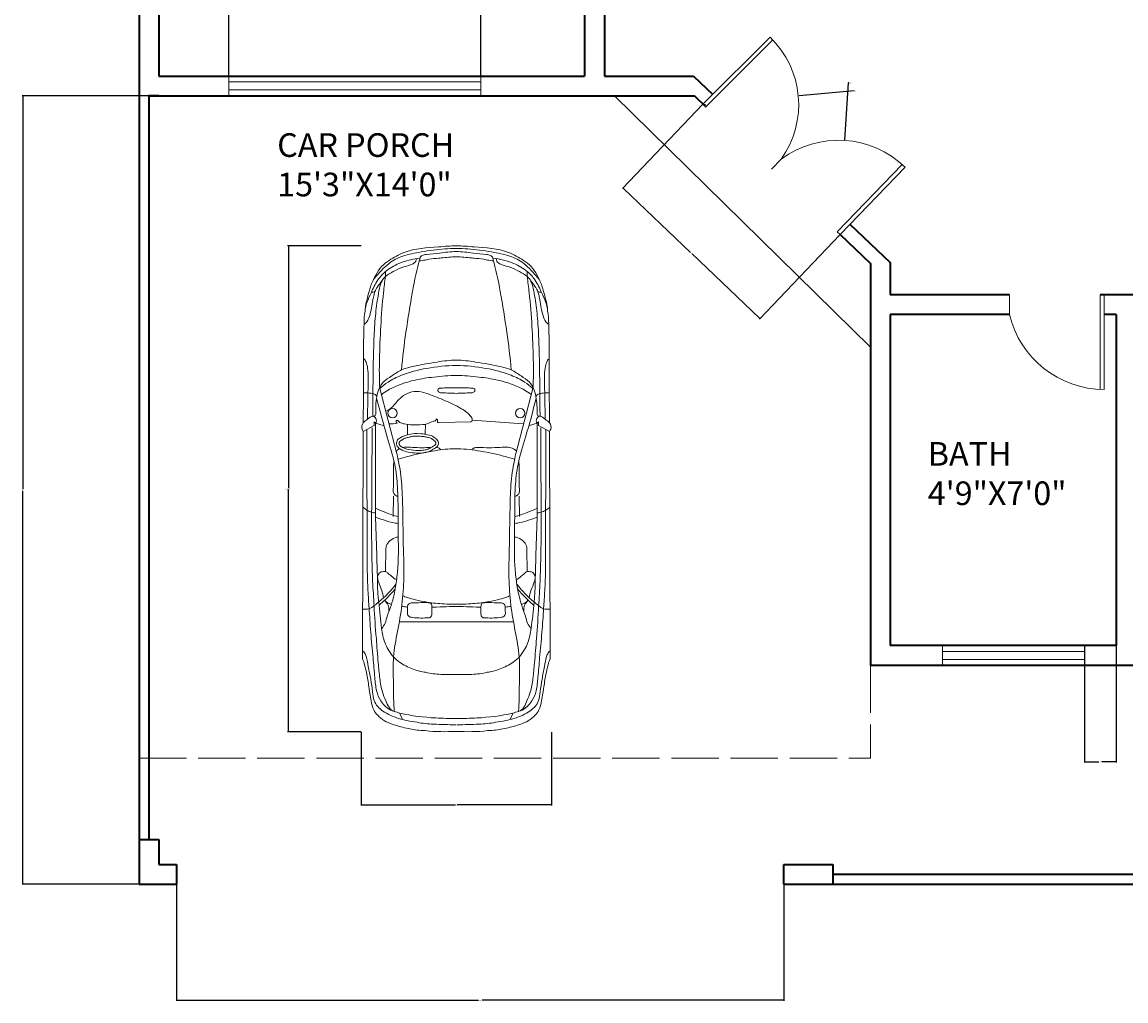
# Model space of a CAD drawing. Units: inches. Extents: x 40921 to 41493, y 89872 to 90511.
# Tile 1 of 4: x 40921 to 41201, y 89872 to 90120. Entities that reach past the tile are written whole.
import ezdxf

# ---------------------------------------------------------------- set-up
doc = ezdxf.new("R2010")
doc.units = ezdxf.units.IN
doc.header["$MEASUREMENT"] = 0
doc.linetypes.add('ACAD_ISO02W100', pattern=[15, 12, -3])
for name, color, linetype, lineweight in [('A-ANNO-DIMS', 2, 'Continuous', 18), ('A-AREA-IDEN', 7, 'Continuous', 18), ('A-DOOR', 3, 'Continuous', 20), ('A-EQPM-VEHC', 8, 'Continuous', 13), ('A-FLOR-STRS', 7, 'Continuous', 18), ('A-GLAZ', 4, 'Continuous', 18), ('A-ROOF-OVHD', 8, 'ACAD_ISO02W100', 13), ('A-WALL', 7, 'Continuous', 35)]:
    doc.layers.add(name, color=color, linetype=linetype, lineweight=lineweight)
doc.styles.get("Standard").update_dxf_attribs({"font": 'arial.ttf'})
doc.dimstyles.get("Standard").update_dxf_attribs({"dimtxt": 0.18, "dimasz": 0.18, "dimexe": 0.18, "dimexo": 0.0625, "dimgap": 0.09, "dimtad": 0, "dimtih": 1, "dimtoh": 1, "dimdec": 4, "dimzin": 0, "dimdsep": 46, "dimtxsty": 'Standard', "dimcen": 0.09, "dimadec": 0, "dimazin": 0, "dimtfac": 1, "dimtdec": 4, "dimtofl": 0, "dimtmove": 0, "dimatfit": 3, "dimfxl": 1, "dimtolj": 1, "dimtzin": 0, "dimarcsym": 0})

# ---------------------------------------------------------------- blocks, each defined once
blk = doc.blocks.new('A$C242571DA')
for p, q in [((1714, 1733), (3817, 1740)), ((1638, 1619), (1625, 1632)), ((1625, 1632), (1660, 1632)), ((1660, 1632), (1714, 1733)), ((1682, 1652), (2695, 1655)), ((1700, 1699), (2985, 1696)), ((1317, 1580), (1910, 1425)), ((1638, 1619), (2503, 1619)), ((1660, 1548), (1638, 1619)), ((2503, 1619), (2862, 1608)), ((1644, 1489), (1610, 1020)), ((2312, 1454), (2501, 1457)), ((3007, 1527), (2808, 1525)), ((3475, 1401), (3475, 843)), ((4315, 1398), (4377, 1370)), ((1626, 1007), (1633, 720)), ((3475, 346), (3475, 904)), ((1740, 585), (1649, 587)), ((1746, 421), (1649, 421)), ((1317, 167), (1910, 322)), ((4315, 349), (4377, 376)), ((2312, 292), (2501, 290)), ((3007, 220), (2808, 222)), ((1638, 128), (1625, 115)), ((1625, 115), (1660, 115)), ((1660, 199), (1638, 128)), ((1638, 128), (2503, 128)), ((1660, 115), (1714, 14)), ((2503, 128), (2862, 139)), ((1682, 95), (2695, 91)), ((1700, 47), (2985, 51)), ((1714, 14), (3817, 7))]:
    blk.add_line(p, q)
for centre in [(1546, 1463), (1546, 284)]:
    blk.add_ellipse(centre, major_axis=(0, 42.9), ratio=0.983266, start_param=4.712389, end_param=10.995574)
for points, knots in [([(605, 1716), (642, 1723), (789, 1729), (1039, 1732), (1344, 1730), (1542, 1733), (1634, 1734)], [0, 0, 0, 0, 0.114897, 0.437061, 0.754269, 1.029686, 1.029686, 1.029686, 1.029686]), ([(1714, 1733), (1708, 1738), (1683, 1753), (1629, 1741), (1606, 1691), (1562, 1652), (1594, 1610), (1628, 1608), (1638, 1619)], [0, 0, 0, 0, 0.024864, 0.0846267, 0.1362471, 0.1900683, 0.2245199, 0.2681841, 0.2681841, 0.2681841, 0.2681841]), ([(2415, 1735), (2425, 1723), (2447, 1699), (2461, 1658), (2468, 1629), (2468, 1616)], [1.808086, 1.808086, 1.808086, 1.808086, 2.918874, 4.131288, 5.10151, 5.10151, 5.10151, 5.10151]), ([(3357, 1739), (3355, 1719), (3361, 1678), (3324, 1632), (3255, 1544), (3187, 1476), (3125, 1432)], [0, 0, 0, 0, 0.0597371, 0.1139981, 0.1672498, 0.3938869, 0.3938869, 0.3938869, 0.3938869]), ([(3745, 1737), (3749, 1730), (3764, 1717), (3811, 1699), (3895, 1687), (4003, 1663), (4108, 1649), (4196, 1638), (4259, 1603), (4302, 1550), (4340, 1484), (4365, 1408), (4390, 1324), (4398, 1267), (4402, 1235)], [0, 0, 0, 0, 0.0219205, 0.0572122, 0.1522539, 0.2718866, 0.3894011, 0.4710097, 0.5346344, 0.5986698, 0.6733118, 0.758696, 0.8351341, 0.9293726, 0.9293726, 0.9293726, 0.9293726]), ([(3817, 1740), (3833, 1730), (3883, 1718), (3973, 1695), (4085, 1680), (4194, 1663), (4281, 1644), (4344, 1598), (4390, 1540), (4427, 1449), (4458, 1337), (4476, 1233), (4478, 1175), (4479, 1162)], [0, 0, 0, 0, 0.056668, 0.14946, 0.28161, 0.392935, 0.481686, 0.542967, 0.622845, 0.69797, 0.833643, 0.965665, 1.00577, 1.00577, 1.00577, 1.00577]), ([(0, 873), (0, 928), (16, 1089), (26, 1310), (121, 1476), (189, 1569), (273, 1623), (370, 1666), (483, 1695), (561, 1715), (605, 1716)], [0, 0, 0, 0, 0.16039, 0.479033, 0.632967, 0.722015, 0.817474, 0.927562, 1.03733, 1.167094, 1.167094, 1.167094, 1.167094]), ([(311, 1637), (282, 1614), (230, 1570), (149, 1486), (85, 1361), (60, 1219), (33, 1054), (25, 945), (25, 873)], [0, 0, 0, 0, 0.1095129, 0.2035347, 0.3452507, 0.5161382, 0.6275464, 0.8383798, 0.8383798, 0.8383798, 0.8383798]), ([(605, 1716), (546, 1714), (449, 1665), (321, 1611), (225, 1521), (147, 1391), (122, 1275), (114, 1209)], [0, 0, 0, 0, 0.1772572, 0.3124951, 0.4151678, 0.5597243, 0.7575412, 0.7575412, 0.7575412, 0.7575412]), ([(427, 1657), (429, 1647), (427, 1625), (400, 1617), (368, 1594), (328, 1565), (272, 1524), (237, 1452), (196, 1377), (184, 1315), (170, 1280), (157, 1254), (133, 1244), (119, 1243)], [0, 0, 0, 0, 0.0304541, 0.0502818, 0.0786089, 0.1479133, 0.1986294, 0.2831705, 0.3780326, 0.4523267, 0.4667809, 0.4902599, 0.5347198, 0.5347198, 0.5347198, 0.5347198]), ([(324, 1558), (345, 1572), (400, 1585), (516, 1607), (680, 1626), (885, 1636), (1117, 1642), (1346, 1644), (1505, 1645), (1574, 1646)], [0, 0, 0, 0, 0.076148, 0.165903, 0.355672, 0.569871, 0.782325, 1.050047, 1.257936, 1.257936, 1.257936, 1.257936]), ([(723, 1727), (721, 1715), (694, 1690), (643, 1672), (574, 1655), (508, 1647), (455, 1635), (429, 1627), (417, 1624)], [0, 0, 0, 0, 0.034703, 0.0959761, 0.1659336, 0.2471559, 0.2929944, 0.3295918, 0.3295918, 0.3295918, 0.3295918]), ([(1044, 1729), (1049, 1718), (1081, 1704), (1139, 1688), (1238, 1686), (1395, 1691), (1522, 1692), (1601, 1693)], [0, 0, 0, 0, 0.0364992, 0.0923739, 0.1867837, 0.3273982, 0.5667068, 0.5667068, 0.5667068, 0.5667068]), ([(1357, 1732), (1357, 1713), (1360, 1679), (1364, 1630), (1383, 1614), (1391, 1607)], [0, 0, 0, 0, 1.462159, 2.651105, 3.386321, 3.386321, 3.386321, 3.386321]), ([(1574, 1646), (1573, 1638), (1574, 1622), (1560, 1619), (1555, 1618)], [0, 0, 0, 0, 0.02274132, 0.03717479, 0.03717479, 0.03717479, 0.03717479]), ([(2695, 1655), (2830, 1655), (3041, 1651), (3351, 1631), (3527, 1623), (3627, 1612)], [0, 0, 0, 0, 0.4042759, 0.6333827, 0.9326252, 0.9326252, 0.9326252, 0.9326252]), ([(2985, 1696), (3051, 1696), (3172, 1691), (3367, 1678), (3575, 1664), (3788, 1644), (3968, 1628), (4104, 1617), (4204, 1578), (4272, 1519), (4301, 1452), (4342, 1305), (4362, 1111), (4367, 937), (4367, 873)], [0, 0, 0, 0, 0.198873, 0.363323, 0.587433, 0.823543, 1.004622, 1.129816, 1.230113, 1.320655, 1.388577, 1.443334, 1.771447, 1.958652, 1.958652, 1.958652, 1.958652]), ([(1317, 1580), (1228, 1586), (1036, 1585), (741, 1573), (486, 1553), (333, 1534), (283, 1528)], [0, 0, 0, 0, 0.269375, 0.574535, 0.885339, 1.036319, 1.036319, 1.036319, 1.036319]), ([(1555, 1618), (1528, 1618), (1473, 1620), (1393, 1609), (1318, 1591), (1249, 1545), (1201, 1467), (1143, 1386), (1105, 1240), (1076, 1072), (1056, 932), (1056, 873)], [0, 0, 0, 0, 0.082256, 0.165174, 0.241383, 0.30939, 0.405348, 0.511507, 0.603349, 0.843635, 1.017671, 1.017671, 1.017671, 1.017671]), ([(1317, 1580), (1297, 1556), (1248, 1494), (1178, 1350), (1124, 1137), (1106, 965), (1106, 873)], [0, 0, 0, 0, 0.0947759, 0.2311242, 0.4700259, 0.7400315, 0.7400315, 0.7400315, 0.7400315]), ([(1373, 1563), (1357, 1545), (1322, 1490), (1277, 1386), (1233, 1244), (1211, 1069), (1197, 942), (1197, 873)], [0, 0, 0, 0, 0.0708922, 0.1925846, 0.3348457, 0.5072814, 0.7109928, 0.7109928, 0.7109928, 0.7109928]), ([(3536, 1563), (3520, 1551), (3484, 1526), (3408, 1511), (3323, 1473), (3208, 1445), (3073, 1422), (2867, 1405), (2626, 1413), (2397, 1411), (2201, 1417), (2001, 1438), (1732, 1526), (1528, 1579), (1408, 1611)], [0, 0, 0, 0, 0.05975, 0.126928, 0.230034, 0.336675, 0.482225, 0.641324, 0.954906, 1.203173, 1.330375, 1.542773, 1.802261, 2.175545, 2.175545, 2.175545, 2.175545]), ([(2424, 1619), (2442, 1590), (2464, 1519), (2495, 1451), (2502, 1411)], [0, 0, 0, 0, 0.1000351, 0.2184418, 0.2184418, 0.2184418, 0.2184418]), ([(2508, 1618), (2521, 1588), (2537, 1527), (2560, 1458), (2563, 1421), (2564, 1411)], [0, 0, 0, 0, 2.528586, 4.711885, 5.408215, 5.408215, 5.408215, 5.408215]), ([(2862, 1608), (2921, 1607), (3047, 1601), (3191, 1602), (3357, 1584), (3498, 1571), (3623, 1549), (3664, 1533)], [0, 0, 0, 0, 0.1783018, 0.3787173, 0.431954, 0.6762374, 0.8077184, 0.8077184, 0.8077184, 0.8077184]), ([(3248, 1545), (3227, 1550), (3176, 1562), (3114, 1593), (3053, 1605), (3010, 1579), (3010, 1545), (3010, 1516), (3034, 1500), (3053, 1465), (3079, 1444), (3084, 1424)], [0, 0, 0, 0, 0.0655106, 0.1550445, 0.2094604, 0.2438604, 0.287164, 0.3001388, 0.3275984, 0.3616951, 0.4200969, 0.4200969, 0.4200969, 0.4200969]), ([(3319, 1587), (3303, 1568), (3257, 1517), (3207, 1467), (3171, 1440)], [0, 0, 0, 0, 1.868162, 5.271297, 5.271297, 5.271297, 5.271297]), ([(3275, 1533), (3288, 1528), (3300, 1505), (3308, 1482), (3312, 1473)], [0, 0, 0, 0, 0.983949, 1.771691, 1.771691, 1.771691, 1.771691]), ([(3372, 1495), (3354, 1497), (3316, 1495), (3292, 1526), (3275, 1533)], [0, 0, 0, 0, 0.0535488, 0.1060573, 0.1060573, 0.1060573, 0.1060573]), ([(3627, 1612), (3702, 1609), (3826, 1597), (3991, 1583), (4112, 1562), (4212, 1523), (4290, 1488), (4301, 1448)], [0, 0, 0, 0, 0.2277977, 0.3719478, 0.4996814, 0.5863441, 0.709615, 0.709615, 0.709615, 0.709615]), ([(3664, 1533), (3687, 1526), (3735, 1502), (3817, 1445), (3884, 1343), (3925, 1240), (3937, 1177), (3940, 1158)], [0, 0, 0, 0, 0.0720749, 0.1581284, 0.2958089, 0.4262456, 0.4842292, 0.4842292, 0.4842292, 0.4842292]), ([(1910, 1425), (1933, 1419), (1996, 1408), (2094, 1386), (2212, 1377), (2419, 1367), (2705, 1366), (3033, 1354), (3316, 1371), (3559, 1416), (3789, 1462), (4029, 1453), (4196, 1455), (4293, 1448), (4301, 1448)], [0, 0, 0, 0, 0.073325, 0.188896, 0.303039, 0.425821, 0.811242, 1.159737, 1.41058, 1.660623, 1.899627, 2.11145, 2.377727, 2.401703, 2.401703, 2.401703, 2.401703]), ([(1997, 1450), (2040, 1455), (2127, 1452), (2220, 1454), (2287, 1457), (2306, 1434), (2313, 1420), (2316, 1414)], [0, 0, 0, 0, 3.267856, 6.568708, 7.399663, 8.099385, 8.621705, 8.621705, 8.621705, 8.621705]), ([(2808, 1525), (2792, 1525), (2752, 1520), (2711, 1473), (2690, 1431), (2691, 1410)], [0, 0, 0, 0, 0.0486628, 0.1144515, 0.1777721, 0.1777721, 0.1777721, 0.1777721]), ([(114, 1209), (215, 1239), (443, 1285), (788, 1339), (1030, 1371), (1146, 1379)], [0, 0, 0, 0, 0.317374, 0.69576, 1.04714, 1.04714, 1.04714, 1.04714]), ([(1898, 1426), (1889, 1421), (1871, 1397), (1856, 1345), (1868, 1234), (1864, 1132), (1863, 1038), (1877, 1022), (1885, 1016)], [0, 0, 0, 0, 0.842998, 2.122875, 3.997599, 9.174838, 10.012722, 10.751336, 10.751336, 10.751336, 10.751336]), ([(1970, 1407), (1960, 1370), (1927, 1259), (1891, 1078), (1874, 933), (1874, 864)], [0, 0, 0, 0, 0.1139079, 0.3411539, 0.543502, 0.543502, 0.543502, 0.543502]), ([(3232, 1368), (3241, 1356), (3253, 1316), (3272, 1241), (3298, 1128), (3311, 975), (3311, 858), (3312, 794)], [0, 0, 0, 0, 0.0451009, 0.1211996, 0.2308505, 0.385263, 0.5739042, 0.5739042, 0.5739042, 0.5739042]), ([(3295, 1175), (3295, 1207), (3300, 1250), (3298, 1304), (3326, 1329), (3364, 1321), (3399, 1329), (3422, 1316), (3431, 1298), (3439, 1234), (3440, 1174), (3435, 1112), (3419, 1102), (3396, 1099), (3363, 1101), (3331, 1097), (3299, 1108), (3297, 1140), (3295, 1161), (3295, 1175)], [0, 0, 0, 0, 0.0969044, 0.1295913, 0.1506192, 0.1985921, 0.2360698, 0.2557908, 0.2719711, 0.2929882, 0.44406, 0.4519132, 0.4720918, 0.4918599, 0.5228758, 0.5707096, 0.5892096, 0.6145759, 0.654681, 0.654681, 0.654681, 0.654681]), ([(4402, 1235), (4412, 1185), (4422, 1066), (4424, 946), (4424, 878)], [0, 0, 0, 0, 0.1502861, 0.3522699, 0.3522699, 0.3522699, 0.3522699]), ([(114, 1209), (103, 1207), (84, 1188), (76, 1122), (68, 1017), (53, 925), (53, 873)], [0, 0, 0, 0, 0.0314754, 0.0702057, 0.1915753, 0.3439346, 0.3439346, 0.3439346, 0.3439346]), ([(136, 1213), (139, 1212), (138, 1193), (133, 1168), (119, 1112), (116, 1059), (109, 975), (102, 920), (102, 873)], [0, 0, 0, 0, 0.0114788, 0.0403472, 0.0875838, 0.1755608, 0.1991501, 0.3369659, 0.3369659, 0.3369659, 0.3369659]), ([(3940, 1158), (3950, 1111), (3964, 1016), (3960, 921), (3960, 873)], [0, 0, 0, 0, 0.140379, 0.2808468, 0.2808468, 0.2808468, 0.2808468]), ([(1311, 873), (1311, 902), (1309, 951), (1315, 1002), (1314, 1039), (1332, 1045), (1346, 1044), (1357, 1029), (1359, 970), (1362, 918), (1363, 873)], [0, 0, 0, 0, 0.0857277, 0.1381048, 0.1641986, 0.1769751, 0.1890325, 0.2028129, 0.2286049, 0.3592554, 0.3592554, 0.3592554, 0.3592554]), ([(1626, 1007), (1623, 1013), (1603, 1029), (1559, 995), (1523, 952), (1480, 878), (1431, 774), (1385, 658), (1344, 551), (1343, 462), (1380, 387), (1428, 330), (1480, 295), (1510, 257), (1525, 233), (1528, 222)], [0, 0, 0, 0, 0.527288, 1.647451, 3.487558, 5.099073, 7.968657, 12.238313, 14.475187, 16.613757, 18.744202, 20.639343, 22.223389, 23.452731, 24.286529, 24.286529, 24.286529, 24.286529]), ([(3339, 1099), (3339, 1095), (3336, 1011), (3333, 926), (3330, 846)], [11.235438, 11.235438, 11.235438, 11.235438, 11.552536, 17.586883, 17.586883, 17.586883, 17.586883]), ([(3232, 379), (3241, 391), (3253, 431), (3272, 506), (3298, 619), (3311, 772), (3311, 888), (3312, 952)], [0, 0, 0, 0, 0.0451009, 0.1211996, 0.2308505, 0.385263, 0.5739042, 0.5739042, 0.5739042, 0.5739042]), ([(0, 873), (0, 819), (16, 658), (26, 437), (121, 270), (189, 178), (273, 124), (370, 80), (483, 52), (561, 32), (605, 31)], [0, 0, 0, 0, 0.16039, 0.479033, 0.632967, 0.722015, 0.817474, 0.927562, 1.03733, 1.167094, 1.167094, 1.167094, 1.167094]), ([(311, 109), (282, 133), (230, 177), (149, 261), (85, 385), (60, 528), (33, 692), (25, 802), (25, 873)], [0, 0, 0, 0, 0.1095129, 0.2035347, 0.3452507, 0.5161382, 0.6275464, 0.8383798, 0.8383798, 0.8383798, 0.8383798]), ([(114, 538), (103, 540), (84, 559), (76, 625), (68, 729), (53, 822), (53, 873)], [0, 0, 0, 0, 0.0314754, 0.0702057, 0.1915753, 0.3439346, 0.3439346, 0.3439346, 0.3439346]), ([(136, 534), (139, 535), (138, 553), (133, 578), (119, 635), (116, 688), (109, 772), (102, 827), (102, 873)], [0, 0, 0, 0, 0.0114788, 0.0403472, 0.0875838, 0.1755608, 0.1991501, 0.3369659, 0.3369659, 0.3369659, 0.3369659]), ([(1555, 129), (1528, 129), (1473, 126), (1393, 138), (1318, 156), (1249, 201), (1201, 280), (1143, 361), (1105, 506), (1076, 674), (1056, 814), (1056, 873)], [0, 0, 0, 0, 0.082256, 0.165174, 0.241383, 0.30939, 0.405348, 0.511507, 0.603349, 0.843635, 1.017671, 1.017671, 1.017671, 1.017671]), ([(1317, 167), (1297, 191), (1248, 252), (1178, 396), (1124, 609), (1106, 782), (1106, 873)], [0, 0, 0, 0, 0.0947759, 0.2311242, 0.4700259, 0.7400315, 0.7400315, 0.7400315, 0.7400315]), ([(1373, 184), (1357, 202), (1322, 257), (1277, 361), (1233, 503), (1211, 677), (1197, 804), (1197, 873)], [0, 0, 0, 0, 0.0708922, 0.1925846, 0.3348457, 0.5072814, 0.7109928, 0.7109928, 0.7109928, 0.7109928]), ([(1311, 873), (1311, 844), (1309, 796), (1315, 745), (1314, 707), (1332, 702), (1346, 703), (1357, 718), (1359, 777), (1362, 829), (1363, 873)], [0, 0, 0, 0, 0.0857277, 0.1381048, 0.1641986, 0.1769751, 0.1890325, 0.2028129, 0.2286049, 0.3592554, 0.3592554, 0.3592554, 0.3592554]), ([(1970, 339), (1960, 377), (1927, 488), (1893, 663), (1874, 802), (1874, 864)], [0, 0, 0, 0, 0.1139079, 0.3411539, 0.5260188, 0.5260188, 0.5260188, 0.5260188]), ([(2985, 51), (3051, 51), (3172, 56), (3367, 69), (3575, 82), (3788, 103), (3968, 119), (4104, 130), (4204, 169), (4272, 227), (4301, 295), (4342, 441), (4362, 636), (4367, 810), (4367, 873)], [0, 0, 0, 0, 0.198873, 0.363323, 0.587433, 0.823543, 1.004622, 1.129816, 1.230113, 1.320655, 1.388577, 1.443334, 1.771447, 1.958652, 1.958652, 1.958652, 1.958652]), ([(3339, 648), (3339, 652), (3336, 736), (3333, 820), (3330, 901)], [11.235438, 11.235438, 11.235438, 11.235438, 11.552536, 17.586883, 17.586883, 17.586883, 17.586883]), ([(3940, 589), (3950, 636), (3964, 730), (3960, 826), (3960, 873)], [0, 0, 0, 0, 0.140379, 0.2808468, 0.2808468, 0.2808468, 0.2808468]), ([(4402, 512), (4412, 561), (4422, 681), (4424, 800), (4424, 869)], [0, 0, 0, 0, 0.1502861, 0.3522699, 0.3522699, 0.3522699, 0.3522699]), ([(1639, 326), (1635, 324), (1629, 318), (1613, 315), (1612, 324), (1613, 330), (1619, 338), (1629, 346), (1638, 366), (1649, 405), (1656, 473), (1656, 543), (1645, 611), (1623, 651), (1615, 684), (1598, 691), (1604, 697), (1610, 700), (1619, 699), (1626, 701), (1638, 699), (1633, 713), (1633, 720)], [0, 0, 0, 0, 0.0138597, 0.0278304, 0.0329137, 0.0379971, 0.0465756, 0.0592704, 0.0762214, 0.1105991, 0.1789801, 0.2766959, 0.3173629, 0.3800771, 0.4110544, 0.4160421, 0.4210284, 0.4277212, 0.4387433, 0.4448131, 0.4508005, 0.4694463, 0.4694463, 0.4694463, 0.4694463]), ([(1863, 686), (1864, 694), (1865, 711), (1877, 724), (1885, 731)], [9.436432, 9.436432, 9.436432, 9.436432, 10.012722, 10.751336, 10.751336, 10.751336, 10.751336]), ([(1740, 585), (1738, 572), (1750, 644), (1766, 664), (1792, 700), (1821, 710), (1853, 704), (1874, 668), (1905, 623), (1916, 557), (1915, 484), (1906, 418), (1885, 363), (1859, 329), (1831, 318), (1811, 323), (1792, 329), (1778, 350), (1753, 386), (1738, 466), (1729, 497), (1742, 598), (1740, 585)], [0, 0, 0, 0, 0.03969, 0.089634, 0.13125, 0.1542862, 0.1797268, 0.2207266, 0.2680991, 0.3447665, 0.4095645, 0.4843001, 0.541515, 0.5817687, 0.6060665, 0.6262474, 0.6436722, 0.6634686, 0.6988791, 0.7758465, 0.8696394, 0.907731, 0.907731, 0.907731, 0.907731]), ([(1765, 587), (1766, 591), (1766, 595), (1769, 606), (1770, 611), (1773, 627), (1776, 633), (1780, 642), (1782, 645), (1786, 651), (1787, 653), (1793, 660), (1797, 666), (1804, 674), (1807, 676), (1811, 679), (1813, 680), (1817, 682), (1819, 683), (1824, 683), (1828, 683), (1832, 682), (1834, 682), (1836, 680), (1838, 679), (1842, 674), (1845, 670), (1850, 662), (1853, 657), (1859, 647), (1862, 643), (1868, 633), (1871, 627), (1877, 616), (1879, 610), (1883, 597), (1884, 591), (1888, 571), (1890, 556), (1891, 527), (1891, 513), (1889, 470), (1885, 441), (1874, 404), (1871, 394), (1863, 379), (1861, 373), (1854, 364), (1851, 359), (1845, 353), (1842, 350), (1836, 346), (1833, 345), (1829, 345), (1828, 345), (1825, 345), (1823, 345), (1818, 346), (1815, 347), (1811, 349), (1809, 349), (1808, 350), (1808, 350), (1807, 351), (1807, 352), (1805, 354), (1803, 356), (1800, 361), (1798, 364), (1795, 368), (1793, 370), (1789, 377), (1787, 381), (1782, 389), (1780, 394), (1777, 403), (1775, 408), (1771, 423), (1768, 434), (1765, 450), (1764, 456), (1761, 467), (1760, 471), (1758, 484), (1757, 493), (1758, 511), (1758, 516), (1759, 528), (1759, 534), (1761, 554), (1763, 571), (1764, 581), (1765, 583), (1765, 585), (1765, 585), (1765, 586), (1765, 587), (1765, 587)], [0.497033, 0.497033, 0.497033, 0.497033, 0.723444, 0.723444, 0.974636, 0.974636, 1.50964, 1.50964, 2.044645, 2.044645, 2.271061, 2.271061, 2.862376, 2.862376, 3.217654, 3.217654, 3.537253, 3.537253, 3.856852, 3.856852, 4.368613, 4.368613, 4.584627, 4.584627, 4.99269, 4.99269, 5.400753, 5.400753, 5.808816, 5.808816, 6.216879, 6.216879, 6.778716, 6.778716, 7.350371, 7.350371, 7.922025, 7.922025, 9.065335, 9.065335, 10.208644, 10.208644, 12.495263, 12.495263, 13.409896, 13.409896, 13.929088, 13.929088, 14.44828, 14.44828, 14.909885, 14.909885, 15.371489, 15.371489, 15.62524, 15.62524, 15.87899, 15.87899, 16.120875, 16.120875, 16.36276, 16.36276, 16.51635, 16.51635, 16.669941, 16.669941, 16.921521, 16.921521, 17.136676, 17.136676, 17.351831, 17.351831, 17.782142, 17.782142, 18.204974, 18.204974, 18.627807, 18.627807, 19.473473, 19.473473, 19.978923, 19.978923, 20.484372, 20.484372, 21.475119, 21.475119, 21.859144, 21.859144, 22.162884, 22.162884, 22.770362, 22.770362, 22.900493, 22.900493, 22.951221, 22.951221, 22.964298, 22.964298, 22.964298, 22.964298]), ([(1864, 379), (1863, 384), (1858, 414), (1867, 502), (1865, 581), (1864, 639)], [1.749253, 1.749253, 1.749253, 1.749253, 2.122875, 3.997599, 8.307432, 8.307432, 8.307432, 8.307432]), ([(3295, 572), (3295, 539), (3300, 497), (3298, 443), (3326, 418), (3364, 426), (3399, 417), (3422, 431), (3431, 449), (3439, 513), (3440, 572), (3435, 635), (3419, 645), (3396, 648), (3363, 646), (3331, 650), (3299, 639), (3297, 606), (3295, 586), (3295, 572)], [0, 0, 0, 0, 0.0969044, 0.1295913, 0.1506192, 0.1985921, 0.2360698, 0.2557908, 0.2719711, 0.2929882, 0.44406, 0.4519132, 0.4720918, 0.4918599, 0.5228758, 0.5707096, 0.5892096, 0.6145759, 0.654681, 0.654681, 0.654681, 0.654681]), ([(605, 31), (546, 32), (449, 82), (321, 136), (225, 226), (147, 356), (122, 472), (114, 538)], [0, 0, 0, 0, 0.1772572, 0.3124951, 0.4151678, 0.5597243, 0.7575412, 0.7575412, 0.7575412, 0.7575412]), ([(114, 538), (215, 508), (443, 462), (788, 408), (1030, 376), (1146, 368)], [0, 0, 0, 0, 0.317374, 0.69576, 1.04714, 1.04714, 1.04714, 1.04714]), ([(3664, 214), (3687, 221), (3735, 244), (3817, 302), (3884, 404), (3925, 507), (3937, 570), (3940, 589)], [0, 0, 0, 0, 0.0720749, 0.1581284, 0.2958089, 0.4262456, 0.4842292, 0.4842292, 0.4842292, 0.4842292]), ([(3745, 10), (3749, 17), (3764, 30), (3811, 48), (3895, 60), (4003, 84), (4108, 98), (4196, 108), (4259, 144), (4302, 197), (4340, 263), (4365, 339), (4390, 422), (4398, 480), (4402, 512)], [0, 0, 0, 0, 0.0219205, 0.0572122, 0.1522539, 0.2718866, 0.3894011, 0.4710097, 0.5346344, 0.5986698, 0.6733118, 0.758696, 0.8351341, 0.9293726, 0.9293726, 0.9293726, 0.9293726]), ([(3817, 7), (3833, 17), (3883, 29), (3973, 52), (4085, 66), (4194, 84), (4281, 102), (4344, 149), (4390, 206), (4427, 298), (4458, 410), (4476, 513), (4478, 572), (4479, 585)], [0, 0, 0, 0, 0.056668, 0.14946, 0.28161, 0.392935, 0.481686, 0.542967, 0.622845, 0.69797, 0.833643, 0.965665, 1.00577, 1.00577, 1.00577, 1.00577]), ([(427, 90), (429, 100), (427, 122), (400, 130), (368, 153), (328, 182), (272, 223), (237, 295), (196, 370), (184, 432), (170, 467), (157, 493), (133, 502), (119, 504)], [0, 0, 0, 0, 0.0304541, 0.0502818, 0.0786089, 0.1479133, 0.1986294, 0.2831705, 0.3780326, 0.4523267, 0.4667809, 0.4902599, 0.5347198, 0.5347198, 0.5347198, 0.5347198]), ([(3536, 184), (3520, 196), (3484, 221), (3408, 236), (3323, 274), (3208, 302), (3073, 325), (2867, 342), (2626, 334), (2397, 336), (2201, 330), (2001, 309), (1732, 221), (1528, 168), (1408, 136)], [0, 0, 0, 0, 0.05975, 0.126928, 0.230034, 0.336675, 0.482225, 0.641324, 0.954906, 1.203173, 1.330375, 1.542773, 1.802261, 2.175545, 2.175545, 2.175545, 2.175545]), ([(1898, 321), (1889, 326), (1881, 337), (1875, 348), (1874, 350)], [0, 0, 0, 0, 0.8429982, 0.9626806, 0.9626806, 0.9626806, 0.9626806]), ([(1910, 322), (1933, 328), (1996, 339), (2094, 361), (2212, 370), (2419, 380), (2705, 380), (3033, 393), (3316, 376), (3559, 331), (3789, 285), (4029, 294), (4196, 292), (4293, 299), (4301, 299)], [0, 0, 0, 0, 0.073325, 0.188896, 0.303039, 0.425821, 0.811242, 1.159737, 1.41058, 1.660623, 1.899627, 2.11145, 2.377727, 2.401703, 2.401703, 2.401703, 2.401703]), ([(1997, 296), (2040, 292), (2127, 295), (2220, 292), (2287, 290), (2306, 312), (2313, 327), (2316, 333)], [0, 0, 0, 0, 3.267856, 6.568708, 7.399663, 8.099385, 8.621705, 8.621705, 8.621705, 8.621705]), ([(2424, 128), (2442, 157), (2464, 228), (2495, 296), (2502, 335)], [0, 0, 0, 0, 0.1000351, 0.2184418, 0.2184418, 0.2184418, 0.2184418]), ([(2508, 128), (2521, 159), (2537, 220), (2560, 288), (2563, 326), (2564, 335)], [0, 0, 0, 0, 2.528586, 4.711885, 5.408215, 5.408215, 5.408215, 5.408215]), ([(2808, 222), (2792, 222), (2752, 227), (2711, 274), (2690, 316), (2691, 337)], [0, 0, 0, 0, 0.0486628, 0.1144515, 0.1777721, 0.1777721, 0.1777721, 0.1777721]), ([(3248, 202), (3227, 196), (3176, 185), (3114, 154), (3053, 141), (3010, 168), (3010, 201), (3010, 231), (3034, 247), (3053, 282), (3079, 303), (3084, 322)], [0, 0, 0, 0, 0.0655106, 0.1550445, 0.2094604, 0.2438604, 0.287164, 0.3001388, 0.3275984, 0.3616951, 0.4200969, 0.4200969, 0.4200969, 0.4200969]), ([(3357, 7), (3355, 28), (3361, 69), (3324, 115), (3255, 203), (3187, 271), (3125, 315)], [0, 0, 0, 0, 0.0597371, 0.1139981, 0.1672498, 0.3938869, 0.3938869, 0.3938869, 0.3938869]), ([(3319, 160), (3303, 179), (3257, 230), (3207, 280), (3171, 307)], [0, 0, 0, 0, 1.868162, 5.271297, 5.271297, 5.271297, 5.271297]), ([(1317, 167), (1228, 161), (1036, 162), (741, 174), (486, 193), (333, 212), (283, 218)], [0, 0, 0, 0, 0.269375, 0.574535, 0.885339, 1.036319, 1.036319, 1.036319, 1.036319]), ([(2862, 139), (2921, 139), (3047, 146), (3191, 145), (3357, 163), (3498, 176), (3623, 197), (3664, 214)], [0, 0, 0, 0, 0.1783018, 0.3787173, 0.431954, 0.6762374, 0.8077184, 0.8077184, 0.8077184, 0.8077184]), ([(3275, 214), (3288, 218), (3300, 242), (3308, 264), (3312, 274)], [0, 0, 0, 0, 0.983949, 1.771691, 1.771691, 1.771691, 1.771691]), ([(3372, 251), (3354, 250), (3316, 252), (3292, 221), (3275, 214)], [0, 0, 0, 0, 0.0535488, 0.1060573, 0.1060573, 0.1060573, 0.1060573]), ([(3627, 135), (3702, 138), (3826, 150), (3991, 164), (4112, 184), (4212, 224), (4290, 259), (4301, 299)], [0, 0, 0, 0, 0.2277977, 0.3719478, 0.4996814, 0.5863441, 0.709615, 0.709615, 0.709615, 0.709615]), ([(324, 189), (345, 175), (400, 162), (516, 140), (680, 121), (885, 111), (1117, 105), (1346, 103), (1505, 102), (1574, 101)], [0, 0, 0, 0, 0.076148, 0.165903, 0.355672, 0.569871, 0.782325, 1.050047, 1.257936, 1.257936, 1.257936, 1.257936]), ([(723, 20), (721, 32), (694, 57), (643, 75), (574, 91), (508, 100), (455, 112), (429, 119), (417, 123)], [0, 0, 0, 0, 0.034703, 0.0959761, 0.1659336, 0.2471559, 0.2929944, 0.3295918, 0.3295918, 0.3295918, 0.3295918]), ([(1357, 15), (1357, 34), (1360, 68), (1364, 116), (1383, 133), (1391, 140)], [0, 0, 0, 0, 1.462159, 2.651105, 3.386321, 3.386321, 3.386321, 3.386321]), ([(1574, 101), (1573, 109), (1574, 125), (1560, 128), (1555, 129)], [0, 0, 0, 0, 0.02274132, 0.03717479, 0.03717479, 0.03717479, 0.03717479]), ([(1714, 14), (1708, 9), (1683, -6), (1629, 6), (1606, 55), (1562, 94), (1594, 137), (1628, 138), (1638, 128)], [0, 0, 0, 0, 0.024864, 0.0846267, 0.1362471, 0.1900683, 0.2245199, 0.2681841, 0.2681841, 0.2681841, 0.2681841]), ([(2415, 12), (2425, 24), (2447, 48), (2461, 89), (2468, 118), (2468, 131)], [1.808086, 1.808086, 1.808086, 1.808086, 2.918874, 4.131288, 5.10151, 5.10151, 5.10151, 5.10151]), ([(2695, 91), (2830, 92), (3041, 95), (3351, 116), (3527, 124), (3627, 135)], [0, 0, 0, 0, 0.4042759, 0.6333827, 0.9326252, 0.9326252, 0.9326252, 0.9326252]), ([(605, 31), (642, 23), (789, 18), (1039, 15), (1344, 17), (1542, 14), (1634, 13)], [0, 0, 0, 0, 0.114897, 0.437061, 0.754269, 1.029686, 1.029686, 1.029686, 1.029686]), ([(1044, 18), (1049, 29), (1081, 43), (1139, 59), (1238, 61), (1395, 55), (1522, 54), (1601, 54)], [0, 0, 0, 0, 0.0364992, 0.0923739, 0.1867837, 0.3273982, 0.5667068, 0.5667068, 0.5667068, 0.5667068])]:
    blk.add_open_spline(points, degree=3, knots=knots)
for points in [[(283, 1528), (268, 1525), (251, 1528), (235, 1528)], [(3332, 1378), (3334, 1360), (3336, 1342), (3337, 1325)], [(4479, 1162), (4491, 1066), (4488, 969), (4488, 873)], [(4479, 585), (4491, 681), (4488, 777), (4488, 873)], [(3332, 369), (3334, 386), (3336, 404), (3337, 422)], [(1646, 253), (1648, 277), (1640, 302), (1639, 326)], [(283, 218), (268, 222), (251, 219), (235, 218)]]:
    blk.add_open_spline(points, degree=3)
blk = doc.blocks.new('DOOR-SWING-24IN')
for p, q in [((3, 0), (3, 24)), ((3, 24), (3, 0)), ((4, 24), (4, 0)), ((27, 0), (27, 5)), ((0, 0), (3, 0)), ((3, 0), (4, 0))]:
    blk.add_line(p, q)
blk.add_arc((3, -0.66), 24.66, 13.265, 90)
blk = doc.blocks.new('WIN-36IN')
for p, q in [((0, 36), (5, 36)), ((0, 0), (0, 36)), ((1.5, 0), (1.5, 36)), ((3.5, 36), (3.5, 0)), ((5, 36), (5, 0)), ((5, 0), (0, 0))]:
    blk.add_line(p, q)
blk = doc.blocks.new('*D17')
at = {"layer": 'A-ANNO-DIMS', "color": 0, "lineweight": -2, "transparency": 16777216}
for p, q in [((41007.46, 90063.57), (40988.84, 90063.57)), ((40989.02, 90063.39), (40989.02, 90002.09)), ((40989.02, 89940.42), (40989.02, 90001.72)), ((41007.46, 89940.24), (40988.84, 89940.24))]:
    blk.add_line(p, q, dxfattribs=at)
at = {"layer": 'A-ANNO-DIMS', "color": 0, "transparency": 16777216}
for points in [[(40988.99, 90063.39), (40989.05, 90063.39), (40989.02, 90063.57)], [(40988.99, 89940.42), (40989.05, 89940.42), (40989.02, 89940.24)]]:
    blk.add_solid(points, dxfattribs=at)
at = {"layer": 'Defpoints', "color": 0, "transparency": 16777216}
for p in [(41007.52, 90063.57), (40989.02, 89940.24), (41007.52, 89940.24)]:
    blk.add_point(p, dxfattribs=at)
at = {"layer": 'A-ANNO-DIMS', "color": 0, "transparency": 16777216, "insert": (40989.02, 90001.9), "char_height": 0.18, "attachment_point": 5}
blk.add_mtext('\\A1;VEHICLE 123', dxfattribs=at)
blk = doc.blocks.new('*D18')
at = {"layer": 'A-ANNO-DIMS', "color": 0, "lineweight": -2, "transparency": 16777216}
for p, q in [((41007.52, 89940.17), (41007.52, 89921.56)), ((41055.72, 89940.17), (41055.72, 89921.56)), ((41007.7, 89921.74), (41031.4, 89921.74)), ((41055.54, 89921.74), (41031.84, 89921.74))]:
    blk.add_line(p, q, dxfattribs=at)
at = {"layer": 'A-ANNO-DIMS', "color": 0, "transparency": 16777216}
for points in [[(41007.7, 89921.77), (41007.7, 89921.71), (41007.52, 89921.74)], [(41055.54, 89921.77), (41055.54, 89921.71), (41055.72, 89921.74)]]:
    blk.add_solid(points, dxfattribs=at)
at = {"layer": 'Defpoints', "color": 0, "transparency": 16777216}
for p in [(41007.52, 89940.24), (41055.72, 89940.24), (41055.72, 89921.74)]:
    blk.add_point(p, dxfattribs=at)
at = {"layer": 'A-ANNO-DIMS', "color": 0, "transparency": 16777216, "insert": (41031.62, 89921.74), "char_height": 0.18, "attachment_point": 5}
blk.add_mtext('\\A1;48', dxfattribs=at)
blk = doc.blocks.new('*D25')
at = {"layer": 'A-ANNO-DIMS', "color": 0, "lineweight": -2, "transparency": 16777216}
for p, q in [((40973.9, 90106.69), (40973.9, 90511.26)), ((40974.08, 90511.08), (41005.48, 90511.08)), ((41037.63, 90511.08), (41006.23, 90511.08)), ((41037.81, 90106.69), (41037.81, 90511.26))]:
    blk.add_line(p, q, dxfattribs=at)
at = {"layer": 'A-ANNO-DIMS', "color": 0, "transparency": 16777216}
for points in [[(40974.08, 90511.11), (40974.08, 90511.05), (40973.9, 90511.08)], [(41037.63, 90511.11), (41037.63, 90511.05), (41037.81, 90511.08)]]:
    blk.add_solid(points, dxfattribs=at)
at = {"layer": 'Defpoints', "color": 0, "transparency": 16777216}
for p in [(41037.81, 90511.08), (40973.9, 90106.63), (41037.81, 90106.63)]:
    blk.add_point(p, dxfattribs=at)
at = {"layer": 'A-ANNO-DIMS', "color": 0, "transparency": 16777216, "insert": (41005.85, 90511.08), "char_height": 0.18, "attachment_point": 5}
blk.add_mtext('\\A1;63.91', dxfattribs=at)
blk = doc.blocks.new('*D26')
at = {"layer": 'A-ANNO-DIMS', "color": 0, "lineweight": -2, "transparency": 16777216}
for p, q in [((40956.15, 90106.69), (40956.15, 90136.26)), ((40956.33, 90136.08), (40964.64, 90136.08)), ((40973.72, 90136.08), (40965.41, 90136.08)), ((40973.9, 90106.69), (40973.9, 90136.26))]:
    blk.add_line(p, q, dxfattribs=at)
at = {"layer": 'A-ANNO-DIMS', "color": 0, "transparency": 16777216}
for points in [[(40956.33, 90136.11), (40956.33, 90136.05), (40956.15, 90136.08)], [(40973.72, 90136.11), (40973.72, 90136.05), (40973.9, 90136.08)]]:
    blk.add_solid(points, dxfattribs=at)
at = {"layer": 'Defpoints', "color": 0, "transparency": 16777216}
for p in [(40973.9, 90136.08), (40956.15, 90106.63), (40973.9, 90106.63)]:
    blk.add_point(p, dxfattribs=at)
at = {"layer": 'A-ANNO-DIMS', "color": 0, "transparency": 16777216, "insert": (40965.02, 90136.08), "char_height": 0.18, "attachment_point": 5}
blk.add_mtext('\\A1;17.75', dxfattribs=at)
blk = doc.blocks.new('*D34')
at = {"layer": 'A-ANNO-DIMS', "color": 0, "lineweight": -2, "transparency": 16777216}
for p, q in [((40960.68, 89901.57), (40960.68, 89872)), ((41114.64, 89901.57), (41114.64, 89872)), ((40960.86, 89872.18), (41037.21, 89872.18)), ((41114.46, 89872.18), (41038.12, 89872.18))]:
    blk.add_line(p, q, dxfattribs=at)
at = {"layer": 'A-ANNO-DIMS', "color": 0, "transparency": 16777216}
for points in [[(40960.86, 89872.21), (40960.86, 89872.15), (40960.68, 89872.18)], [(41114.46, 89872.21), (41114.46, 89872.15), (41114.64, 89872.18)]]:
    blk.add_solid(points, dxfattribs=at)
at = {"layer": 'Defpoints', "color": 0, "transparency": 16777216}
for p in [(40960.68, 89901.63), (41114.64, 89901.63), (41114.64, 89872.18)]:
    blk.add_point(p, dxfattribs=at)
at = {"layer": 'A-ANNO-DIMS', "color": 0, "transparency": 16777216, "insert": (41037.66, 89872.18), "char_height": 0.18, "attachment_point": 5}
blk.add_mtext('\\A1;153.96', dxfattribs=at)
blk = doc.blocks.new('*D35')
at = {"layer": 'A-ANNO-DIMS', "color": 0, "lineweight": -2, "transparency": 16777216}
for p, q in [((40953.59, 90101.63), (40921.52, 90101.63)), ((40921.7, 90101.45), (40921.7, 90001.81)), ((40921.7, 89901.81), (40921.7, 90001.45)), ((40951.09, 89901.63), (40921.52, 89901.63))]:
    blk.add_line(p, q, dxfattribs=at)
at = {"layer": 'A-ANNO-DIMS', "color": 0, "transparency": 16777216}
for points in [[(40921.67, 90101.45), (40921.73, 90101.45), (40921.7, 90101.63)], [(40921.67, 89901.81), (40921.73, 89901.81), (40921.7, 89901.63)]]:
    blk.add_solid(points, dxfattribs=at)
at = {"layer": 'Defpoints', "color": 0, "transparency": 16777216}
for p in [(40921.7, 90101.63), (40953.65, 90101.63), (40951.15, 89901.63)]:
    blk.add_point(p, dxfattribs=at)
at = {"layer": 'A-ANNO-DIMS', "color": 0, "transparency": 16777216, "insert": (40921.7, 90001.63), "char_height": 0.18, "attachment_point": 5}
blk.add_mtext('\\A1;200', dxfattribs=at)
blk = doc.blocks.new('*D41')
at = {"layer": 'A-ANNO-DIMS', "color": 0, "lineweight": -2, "transparency": 16777216}
for p, q in [((41190.86, 89962.07), (41190.86, 89932.5)), ((41198.9, 89962.07), (41198.9, 89932.5)), ((41191.04, 89932.68), (41194.5, 89932.68)), ((41198.72, 89932.68), (41195.26, 89932.68))]:
    blk.add_line(p, q, dxfattribs=at)
at = {"layer": 'A-ANNO-DIMS', "color": 0, "transparency": 16777216}
for points in [[(41191.04, 89932.71), (41191.04, 89932.65), (41190.86, 89932.68)], [(41198.72, 89932.71), (41198.72, 89932.65), (41198.9, 89932.68)]]:
    blk.add_solid(points, dxfattribs=at)
at = {"layer": 'Defpoints', "color": 0, "transparency": 16777216}
for p in [(41190.86, 89962.13), (41198.9, 89962.13), (41190.86, 89932.68)]:
    blk.add_point(p, dxfattribs=at)
at = {"layer": 'A-ANNO-DIMS', "color": 0, "transparency": 16777216, "insert": (41194.88, 89932.68), "char_height": 0.18, "attachment_point": 5}
blk.add_mtext('\\A1;8.041', dxfattribs=at)
blk = doc.blocks.new('*D43')
at = {"layer": 'A-ANNO-DIMS', "color": 0, "lineweight": -2, "transparency": 16777216}
for p, q in [((41094.13, 90099.51), (41073.73, 90078.12)), ((41073.98, 90078.12), (41091.03, 90061.87)), ((41128.87, 90066.39), (41108.47, 90044.99)), ((41108.46, 90045.25), (41091.41, 90061.5))]:
    blk.add_line(p, q, dxfattribs=at)
at = {"layer": 'A-ANNO-DIMS', "color": 0, "transparency": 16777216}
for points in [[(41074, 90078.14), (41073.96, 90078.1), (41073.85, 90078.25)], [(41108.48, 90045.27), (41108.44, 90045.22), (41108.59, 90045.12)]]:
    blk.add_solid(points, dxfattribs=at)
at = {"layer": 'Defpoints', "color": 0, "transparency": 16777216}
for p in [(41094.18, 90099.56), (41073.85, 90078.25), (41128.92, 90066.44)]:
    blk.add_point(p, dxfattribs=at)
at = {"layer": 'A-ANNO-DIMS', "color": 0, "transparency": 16777216, "insert": (41091.22, 90061.68), "char_height": 0.18, "attachment_point": 5}
blk.add_mtext('\\A1;48', dxfattribs=at)
blk = doc.blocks.new('*D48')
at = {"layer": 'A-ANNO-DIMS', "color": 0, "lineweight": -2, "transparency": 16777216}
for p, q in [((41130.99, 90104.89), (41130.06, 90090.48)), ((41131.17, 90104.89), (41130.99, 90104.89)), ((41128.4, 90065.99), (41128.58, 90065.99)), ((41128.49, 90065.9), (41128.49, 90066.08))]:
    blk.add_line(p, q, dxfattribs=at)
at = {"layer": 'A-ANNO-DIMS', "color": 0, "transparency": 16777216}
blk.add_solid([(41130.03, 90090.49), (41130.09, 90090.48), (41130.05, 90090.3)], dxfattribs=at)
at = {"layer": 'Defpoints', "color": 0, "transparency": 16777216}
for p in [(41130.05, 90090.3), (41128.49, 90065.99)]:
    blk.add_point(p, dxfattribs=at)
at = {"layer": 'A-ANNO-DIMS', "color": 0, "transparency": 16777216, "insert": (41131.72, 90104.89), "char_height": 0.18, "attachment_point": 5}
blk.add_mtext('\\A1;R24.365', dxfattribs=at)
blk = doc.blocks.new('*D49')
at = {"layer": 'A-ANNO-DIMS', "color": 0, "lineweight": -2, "transparency": 16777216}
for p, q in [((41132.53, 90102.85), (41118.51, 90101.58)), ((41094.58, 90099.41), (41094.76, 90099.41)), ((41094.67, 90099.32), (41094.67, 90099.5))]:
    blk.add_line(p, q, dxfattribs=at)
at = {"layer": 'A-ANNO-DIMS', "color": 0, "transparency": 16777216}
blk.add_solid([(41118.51, 90101.61), (41118.51, 90101.55), (41118.33, 90101.56)], dxfattribs=at)
at = {"layer": 'Defpoints', "color": 0, "transparency": 16777216}
for p in [(41118.33, 90101.56), (41094.67, 90099.41)]:
    blk.add_point(p, dxfattribs=at)
at = {"layer": 'A-ANNO-DIMS', "color": 0, "transparency": 16777216, "insert": (41133.08, 90102.85), "char_height": 0.18, "attachment_point": 5}
blk.add_mtext('\\A1;R23.756', dxfattribs=at)

msp = doc.modelspace()

# ---------------------------------------------------------------- linework, layer by layer
at = {"layer": 'A-DOOR'}
for p, q in [((41094.1751, 90099.5601), (41111.155, 90116.5213)), ((41094.8818, 90098.8526), (41111.8617, 90115.8138)), ((41092.0036, 90101.6306), (41094.1545, 90099.5393)), ((41094.1545, 90099.5393), (41094.1751, 90099.5601)), ((41094.1751, 90099.5601), (41094.8991, 90098.8698)), ((41094.1751, 90099.5601), (41094.1751, 90099.5601)), ((41111.5446, 90082.9986), (41113.9675, 90085.5554)), ((41144.6724, 90084.2295), (41128.1951, 90067.1301)), ((41128.9152, 90066.4362), (41145.3924, 90083.5356)), ((41145.3924, 90083.5356), (41128.9152, 90066.4362)), ((41128.9152, 90066.4362), (41128.1951, 90067.1301))]:
    msp.add_line(p, q, dxfattribs=at)
for centre, radius, start, end in [((41094.6728, 90099.4137), 23.7558, 324.312557, 46.066709), ((41128.4872, 90065.9889), 24.3654, 46.066709, 126.578091)]:
    msp.add_arc(centre, radius, start, end, dxfattribs=at)
at = {"layer": 'A-FLOR-STRS'}
msp.add_line((41071.7434, 90101.6306), (41136.6503, 90037.8699), dxfattribs=at)
at = {"layer": 'A-GLAZ'}
for p, q in [((40973.8989, 90106.6306), (40973.8989, 90101.6306)), ((41037.8072, 90106.6306), (40973.8989, 90106.6306)), ((41037.8072, 90105.1306), (40973.8989, 90105.1306)), ((41037.8072, 90101.6306), (41037.8072, 90106.6306)), ((40973.8989, 90103.1306), (40977.8072, 90103.1306)), ((40973.8989, 90101.6306), (40977.8072, 90101.6306)), ((40977.8072, 90103.1306), (41037.8072, 90103.1306)), ((40977.8072, 90101.6306), (41037.8072, 90101.6306)), ((41154.8592, 89962.1306), (41154.8592, 89962.1306))]:
    msp.add_line(p, q, dxfattribs=at)
at = {"layer": 'A-ROOF-OVHD'}
for p in [(41136.6503, 89957.1306), (40951.1503, 89933.6306)]:
    msp.add_line(p, (41136.6503, 89933.6306), dxfattribs=at)
at = {"layer": 'A-WALL'}
for p, q in [((40951.1503, 90481.6306), (40951.1503, 89901.6306)), ((40956.1503, 90476.6306), (40956.1503, 90106.6306)), ((41064.1503, 90135.1497), (41064.1503, 90106.6306)), ((41069.1503, 90135.1497), (41069.1503, 90106.6306)), ((40956.1503, 90106.6306), (41064.1503, 90106.6306)), ((41069.1503, 90106.6306), (41091.7272, 90106.6306)), ((41091.7272, 90106.6306), (41096.6158, 90101.9981)), ((40953.6503, 90101.6306), (41092.0036, 90101.6306)), ((40956.1503, 90101.6306), (40953.6503, 90101.6306)), ((40953.6503, 90101.6306), (40953.6503, 89912.9449)), ((41092.0036, 90101.6306), (41094.8991, 90098.8698)), ((41131.4107, 90069.026), (41141.6503, 90059.3228)), ((41128.9152, 90066.4362), (41136.6503, 90059.0609)), ((41141.6503, 90059.3228), (41141.6503, 90051.1306)), ((41136.6503, 90059.0609), (41136.6503, 89957.1306)), ((41171.9003, 90051.1306), (41141.6503, 90051.1306)), ((41261.1503, 90051.1306), (41194.9003, 90051.1306)), ((41171.9003, 90046.1306), (41141.6503, 90046.1306)), ((41141.6503, 90046.1306), (41141.6503, 89962.1306)), ((41198.9003, 90046.1306), (41195.9003, 90046.1306)), ((41198.9003, 90046.1306), (41198.9003, 89962.1306)), ((41198.9003, 89962.1306), (41141.6503, 89962.1306)), ((41261.1503, 89957.1306), (41136.6503, 89957.1306)), ((40951.1503, 89912.9449), (40956.1507, 89912.9449)), ((40956.1507, 89912.9449), (40956.1507, 89906.6306)), ((40956.1507, 89906.6306), (40960.6819, 89906.6306)), ((40960.6819, 89906.6306), (40960.6819, 89901.6306)), ((41114.6387, 89901.6306), (41114.6387, 89906.6306)), ((41114.6387, 89906.6306), (41127.0765, 89906.6306)), ((41127.0765, 89906.6306), (41127.0765, 89901.6306)), ((41127.0765, 89904.1306), (41261.1503, 89904.1306)), ((40951.1503, 89901.6306), (40960.6819, 89901.6306)), ((41114.6387, 89901.6306), (41463.1503, 89901.6306))]:
    msp.add_line(p, q, dxfattribs=at)

# ---------------------------------------------------------------- block references
at = {"layer": 'A-DOOR', "rotation": 180}
msp.add_blockref('DOOR-SWING-24IN', (41198.9006, 90051.1303), dxfattribs=at)
at = {"layer": 'A-EQPM-VEHC', "xscale": 0.0274623664719991, "yscale": 0.0274623664719991, "zscale": 0.0274623664719991, "rotation": 270}
msp.add_blockref('A$C242571DA', (41007.6339, 90063.5712), dxfattribs=at)
at = {"layer": 'A-GLAZ', "rotation": 89.99999999999685}
msp.add_blockref('WIN-36IN', (41190.8588, 89957.1303), dxfattribs=at)

# ---------------------------------------------------------------- texts
at = {"layer": 'A-AREA-IDEN', "char_height": 6, "attachment_point": 1}
for s, width, insert in [('CAR PORCH\\P15\'3"X14\'0"', 73.126256, (40986.1906, 90092.1271)), ('BATH\\P4\'9"X7\'0"', 38.908323, (41151.1625, 90013.7953))]:
    msp.add_mtext_dynamic_manual_height_columns(s, width=width, gutter_width=1, heights=[0], dxfattribs=dict(at, insert=insert))

# ---------------------------------------------------------------- dimensions: what is measured, and where the dimension line sits
at = {"layer": 'A-ANNO-DIMS'}
for base, p1, p2, override, picture, middle in [((41037.8072, 90511.0806), (40973.8989, 90106.6306), (41037.8072, 90106.6306), {"dimdec": 2, "dimlfac": 1, "dimrnd": 0, "dimzin": 0, "dimdsep": 46, "dimlunit": 2}, '*D25', (41005.8531, 90511.0806)), ((40973.8989, 90136.0806), (40956.1503, 90106.6306), (40973.8989, 90106.6306), {"dimdec": 2, "dimlfac": 1, "dimrnd": 0, "dimzin": 0, "dimdsep": 46, "dimlunit": 2}, '*D26', (40965.0246, 90136.0806)), ((41055.7169, 89921.7362), (41007.5211, 89940.2364), (41055.7169, 89940.2364), {"dimdec": 0, "dimlfac": 1, "dimrnd": 0, "dimzin": 0, "dimdsep": 46, "dimlunit": 2}, '*D18', (41031.619, 89921.7362)), ((41114.6387, 89872.1806), (40960.6819, 89901.6306), (41114.6387, 89901.6306), {"dimdec": 2, "dimlfac": 1, "dimrnd": 0, "dimzin": 0, "dimdsep": 46, "dimlunit": 2}, '*D34', (41037.6603, 89872.1806))]:
    dim = msp.add_linear_dim(base=base, p1=p1, p2=p2, dimstyle='Standard', override=override, dxfattribs=at)
    dim.commit()
    dim.dimension.update_dxf_attribs({"geometry": picture, "text_midpoint": middle})
for center, mpoint, picture, middle in [((41128.4872, 90065.9889), (41130.05, 90090.3041), '*D48', (41131.7181, 90104.8932)), ((41094.6728, 90099.4137), (41118.3312, 90101.562), '*D49', (41132.5263, 90102.851))]:
    dim = msp.add_radius_dim(center=center, mpoint=mpoint, dimstyle='Standard', override={"dimdec": 3, "dimlfac": 1, "dimrnd": 0, "dimzin": 0, "dimdsep": 46, "dimlunit": 2}, dxfattribs=at)
    dim.commit()
    dim.dimension.update_dxf_attribs({"geometry": picture, "text_midpoint": middle, "dimtype": 164})
for base, p1, p2, angle, override, picture, middle in [((40921.7003, 90101.6306), (40951.1503, 89901.6306), (40953.6503, 90101.6306), 90, {"dimdec": 0, "dimlfac": 1, "dimrnd": 0, "dimzin": 0, "dimdsep": 46, "dimlunit": 2}, '*D35', (40921.7003, 90001.6306)), ((41073.8525, 90078.246), (41128.9152, 90066.4362), (41094.1751, 90099.5601), 136.364198, {"dimdec": 0, "dimlfac": 1, "dimrnd": 0, "dimzin": 0, "dimdsep": 46, "dimlunit": 2}, '*D43', (41091.2225, 90061.684)), ((41190.8592, 89932.6806), (41198.9003, 89962.1306), (41190.8592, 89962.1306), 180, {"dimdec": 3, "dimlfac": 1, "dimrnd": 0, "dimzin": 0, "dimdsep": 46, "dimlunit": 2}, '*D41', (41194.8798, 89932.6806))]:
    dim = msp.add_linear_dim(base=base, p1=p1, p2=p2, angle=angle, dimstyle='Standard', override=override, dxfattribs=at)
    dim.commit()
    dim.dimension.update_dxf_attribs({"geometry": picture, "text_midpoint": middle})
dim = msp.add_linear_dim(base=(40989.0209, 89940.2364), p1=(41007.5211, 90063.5712), p2=(41007.5211, 89940.2364), angle=270, text='VEHICLE <>', dimstyle='Standard', override={"dimdec": 0, "dimlfac": 1, "dimrnd": 0, "dimzin": 0, "dimdsep": 46, "dimlunit": 2}, dxfattribs=at)
dim.commit()
dim.dimension.update_dxf_attribs({"geometry": '*D17', "text_midpoint": (40989.0209, 90001.9038)})

doc.saveas('drawing.dxf')
